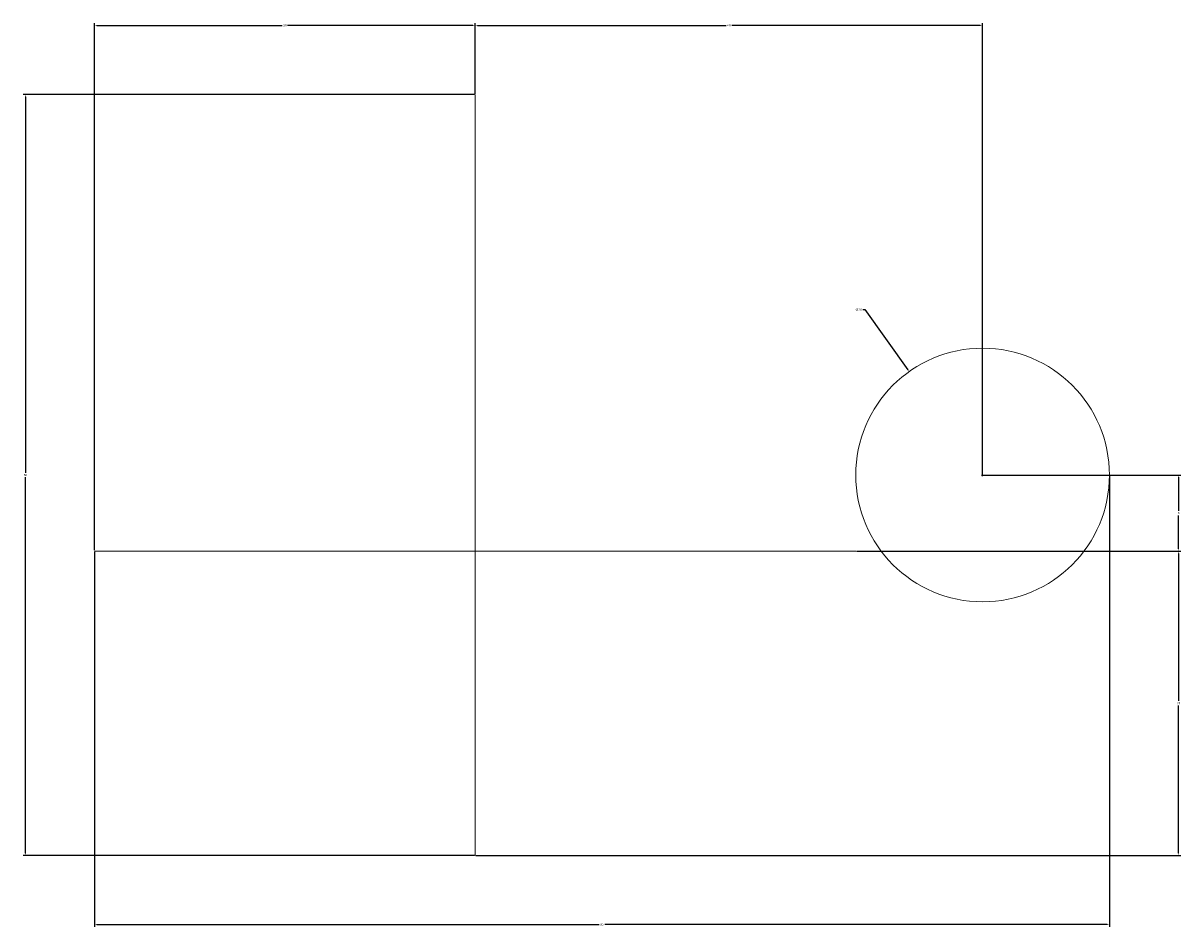
# Model space of a CAD drawing. Units: millimetres. Extents: x 0 to 390, y -312 to 42.
# Tile 3 of 3: x 299 to 390, y -30 to 42. Entities that reach past the tile are written whole.
import ezdxf

# ---------------------------------------------------------------- set-up
doc = ezdxf.new("R2010")
doc.units = ezdxf.units.MM
doc.layers.add('M-CONS', color=8, linetype='Continuous', lineweight=18)
doc.layers.add('M-DIMS', color=2, linetype='Continuous', lineweight=18)
doc.styles.get("Standard").update_dxf_attribs({"font": 'arial.ttf'})
doc.dimstyles.get("Standard").update_dxf_attribs({"dimtxt": 0.18, "dimasz": 0.18, "dimexe": 0.18, "dimexo": 0.0625, "dimgap": 0.09, "dimtad": 0, "dimtih": 1, "dimtoh": 1, "dimdec": 4, "dimzin": 0, "dimdsep": 46, "dimtxsty": 'Standard', "dimcen": 0.09, "dimadec": 0, "dimazin": 0, "dimtfac": 1, "dimtdec": 4, "dimtofl": 0, "dimtmove": 0, "dimatfit": 3, "dimfxl": 1, "dimtolj": 1, "dimtzin": 0, "dimarcsym": 0})

# ---------------------------------------------------------------- blocks, each defined once
blk = doc.blocks.new('*D4')
at = {"layer": 'Defpoints', "color": 0, "transparency": 16777216}
for p in [(384.394, 6), (304.394, 0), (384.394, -29.45)]:
    blk.add_point(p, dxfattribs=at)
at = {"layer": 'M-DIMS', "color": 0, "lineweight": -2, "transparency": 16777216}
for p, q in [((384.394, 5.938), (384.394, -29.63)), ((304.394, -0.062), (304.394, -29.63)), ((304.574, -29.45), (344.175, -29.45)), ((384.214, -29.45), (344.613, -29.45))]:
    blk.add_line(p, q, dxfattribs=at)
at = {"layer": 'M-DIMS', "color": 0, "transparency": 16777216}
for points in [[(304.574, -29.42), (304.574, -29.48), (304.394, -29.45)], [(384.214, -29.42), (384.214, -29.48), (384.394, -29.45)]]:
    blk.add_solid(points, dxfattribs=at)
at = {"layer": 'M-DIMS', "color": 0, "transparency": 16777216, "insert": (344.394, -29.45), "char_height": 0.18, "attachment_point": 5}
blk.add_mtext('\\A1;80', dxfattribs=at)
blk = doc.blocks.new('*D5')
at = {"layer": 'Defpoints', "color": 0, "transparency": 16777216}
for p in [(298.944, 36), (334.394, 36), (334.394, -24)]:
    blk.add_point(p, dxfattribs=at)
at = {"layer": 'M-DIMS', "color": 0, "lineweight": -2, "transparency": 16777216}
for p, q in [((334.332, 36), (298.764, 36)), ((298.944, 35.82), (298.944, 6.182)), ((298.944, -23.82), (298.944, 5.818)), ((334.332, -24), (298.764, -24))]:
    blk.add_line(p, q, dxfattribs=at)
at = {"layer": 'M-DIMS', "color": 0, "transparency": 16777216}
for points in [[(298.914, 35.82), (298.974, 35.82), (298.944, 36)], [(298.914, -23.82), (298.974, -23.82), (298.944, -24)]]:
    blk.add_solid(points, dxfattribs=at)
at = {"layer": 'M-DIMS', "color": 0, "transparency": 16777216, "insert": (298.944, 6), "char_height": 0.18, "attachment_point": 5}
blk.add_mtext('\\A1;60', dxfattribs=at)
blk = doc.blocks.new('*D6')
at = {"layer": 'Defpoints', "color": 0, "transparency": 16777216}
for p in [(334.394, 41.45), (334.394, 36), (304.394, 0)]:
    blk.add_point(p, dxfattribs=at)
at = {"layer": 'M-DIMS', "color": 0, "lineweight": -2, "transparency": 16777216}
for p, q in [((304.394, 0.062), (304.394, 41.63)), ((304.574, 41.45), (319.176, 41.45)), ((334.214, 41.45), (319.613, 41.45)), ((334.394, 36.062), (334.394, 41.63))]:
    blk.add_line(p, q, dxfattribs=at)
at = {"layer": 'M-DIMS', "color": 0, "transparency": 16777216}
for points in [[(304.574, 41.48), (304.574, 41.42), (304.394, 41.45)], [(334.214, 41.48), (334.214, 41.42), (334.394, 41.45)]]:
    blk.add_solid(points, dxfattribs=at)
at = {"layer": 'M-DIMS', "color": 0, "transparency": 16777216, "insert": (319.394, 41.45), "char_height": 0.18, "attachment_point": 5}
blk.add_mtext('\\A1;30', dxfattribs=at)
blk = doc.blocks.new('*D7')
at = {"layer": 'Defpoints', "color": 0, "transparency": 16777216}
for p in [(374.394, 41.45), (334.394, 36), (374.394, 6)]:
    blk.add_point(p, dxfattribs=at)
at = {"layer": 'M-DIMS', "color": 0, "lineweight": -2, "transparency": 16777216}
for p, q in [((334.394, 36.062), (334.394, 41.63)), ((334.574, 41.45), (354.172, 41.45)), ((374.214, 41.45), (354.616, 41.45)), ((374.394, 6.062), (374.394, 41.63))]:
    blk.add_line(p, q, dxfattribs=at)
at = {"layer": 'M-DIMS', "color": 0, "transparency": 16777216}
for points in [[(334.574, 41.48), (334.574, 41.42), (334.394, 41.45)], [(374.214, 41.48), (374.214, 41.42), (374.394, 41.45)]]:
    blk.add_solid(points, dxfattribs=at)
at = {"layer": 'M-DIMS', "color": 0, "transparency": 16777216, "insert": (354.394, 41.45), "char_height": 0.18, "attachment_point": 5}
blk.add_mtext('\\A1;40', dxfattribs=at)
blk = doc.blocks.new('*D8')
at = {"layer": 'Defpoints', "color": 0, "transparency": 16777216}
for p in [(364.394, 0), (389.844, 0), (334.394, -24)]:
    blk.add_point(p, dxfattribs=at)
at = {"layer": 'M-DIMS', "color": 0, "lineweight": -2, "transparency": 16777216}
for p, q in [((364.457, 0), (390.024, 0)), ((389.844, -0.18), (389.844, -11.82)), ((389.844, -23.82), (389.844, -12.18)), ((334.457, -24), (390.024, -24))]:
    blk.add_line(p, q, dxfattribs=at)
at = {"layer": 'M-DIMS', "color": 0, "transparency": 16777216}
for points in [[(389.814, -0.18), (389.874, -0.18), (389.844, 0)], [(389.814, -23.82), (389.874, -23.82), (389.844, -24)]]:
    blk.add_solid(points, dxfattribs=at)
at = {"layer": 'M-DIMS', "color": 0, "transparency": 16777216, "insert": (389.844, -12), "char_height": 0.18, "attachment_point": 5}
blk.add_mtext('\\A1;24', dxfattribs=at)
blk = doc.blocks.new('*D9')
at = {"layer": 'Defpoints', "color": 0, "transparency": 16777216}
for p in [(374.394, 6), (389.844, 6), (364.394, 0)]:
    blk.add_point(p, dxfattribs=at)
at = {"layer": 'M-DIMS', "color": 0, "lineweight": -2, "transparency": 16777216}
for p, q in [((374.457, 6), (390.024, 6)), ((389.844, 5.82), (389.844, 3.182)), ((389.844, 0.18), (389.844, 2.818)), ((364.457, 0), (390.024, 0))]:
    blk.add_line(p, q, dxfattribs=at)
at = {"layer": 'M-DIMS', "color": 0, "transparency": 16777216}
for points in [[(389.814, 5.82), (389.874, 5.82), (389.844, 6)], [(389.814, 0.18), (389.874, 0.18), (389.844, 0)]]:
    blk.add_solid(points, dxfattribs=at)
at = {"layer": 'M-DIMS', "color": 0, "transparency": 16777216, "insert": (389.844, 3), "char_height": 0.18, "attachment_point": 5}
blk.add_mtext('\\A1;6', dxfattribs=at)
blk = doc.blocks.new('*D12')
at = {"layer": 'Defpoints', "color": 0, "transparency": 16777216}
for p in [(368.6, 14.15), (380.188, -2.15)]:
    blk.add_point(p, dxfattribs=at)
at = {"layer": 'M-DIMS', "color": 0, "lineweight": -2, "transparency": 16777216}
for p, q in [((364.943, 19.04), (365.123, 19.04)), ((365.123, 19.04), (368.496, 14.297)), ((374.304, 6), (374.484, 6)), ((374.394, 5.91), (374.394, 6.09))]:
    blk.add_line(p, q, dxfattribs=at)
at = {"layer": 'M-DIMS', "color": 0, "transparency": 16777216}
blk.add_solid([(368.52, 14.314), (368.471, 14.28), (368.6, 14.15)], dxfattribs=at)
at = {"layer": 'M-DIMS', "color": 0, "transparency": 16777216, "insert": (364.627, 19.04), "char_height": 0.18, "attachment_point": 5}
blk.add_mtext('\\A1;∅20', dxfattribs=at)

msp = doc.modelspace()

# ---------------------------------------------------------------- linework, layer by layer
at = {"layer": 'M-CONS'}
msp.add_line((334.394, -24, 343.814), (334.394, 36, 343.814), dxfattribs=at)
at = {"layer": 'M-CONS', "extrusion": (0, -1, 0)}
msp.add_lwpolyline([(334.394, 307.814), (334.394, 343.814), (307.672, 291.45)], dxfattribs=at)
at = {"layer": 'M-CONS'}
msp.add_circle((374.394, 6, 383.814), 10, dxfattribs=at)
at = {"layer": 'M-CONS', "extrusion": (0, -1, 0)}
for radius in [30, 15]:
    msp.add_circle((334.394, 277.814), radius, dxfattribs=at)

# ---------------------------------------------------------------- dimensions: what is measured, and where the dimension line sits
at = {"layer": 'M-DIMS'}
for base, p1, p2, picture, middle in [((334.394, 41.45), (304.394, 0), (334.394, 36), '*D6', (319.394, 41.45)), ((374.394, 41.45), (334.394, 36), (374.394, 6), '*D7', (354.394, 41.45)), ((384.394, -29.45), (304.394, 0), (384.394, 6), '*D4', (344.394, -29.45))]:
    dim = msp.add_linear_dim(base=base, p1=p1, p2=p2, dimstyle='Standard', override={"dimdec": 0, "dimlfac": 1, "dimrnd": 0, "dimzin": 0, "dimdsep": 46, "dimlunit": 2}, dxfattribs=at)
    dim.commit()
    dim.dimension.update_dxf_attribs({"geometry": picture, "text_midpoint": middle})
for base, p1, p2, picture, middle in [((298.944, 36), (334.394, -24), (334.394, 36), '*D5', (298.944, 6)), ((389.844, 6), (364.394, 0), (374.394, 6), '*D9', (389.844, 3)), ((389.844, 0), (334.394, -24), (364.394, 0), '*D8', (389.844, -12))]:
    dim = msp.add_linear_dim(base=base, p1=p1, p2=p2, angle=90, dimstyle='Standard', override={"dimdec": 0, "dimlfac": 1, "dimrnd": 0, "dimzin": 0, "dimdsep": 46, "dimlunit": 2}, dxfattribs=at)
    dim.commit()
    dim.dimension.update_dxf_attribs({"geometry": picture, "text_midpoint": middle})
dim = msp.add_diameter_dim_2p(p1=(380.188, -2.15), p2=(368.6, 14.15), dimstyle='Standard', override={"dimdec": 0, "dimlfac": 1, "dimrnd": 0, "dimzin": 0, "dimdsep": 46, "dimlunit": 2}, dxfattribs=at)
dim.commit()
dim.dimension.update_dxf_attribs({"geometry": '*D12', "text_midpoint": (364.627, 19.04), "dimtype": 163})

doc.saveas('drawing.dxf')
